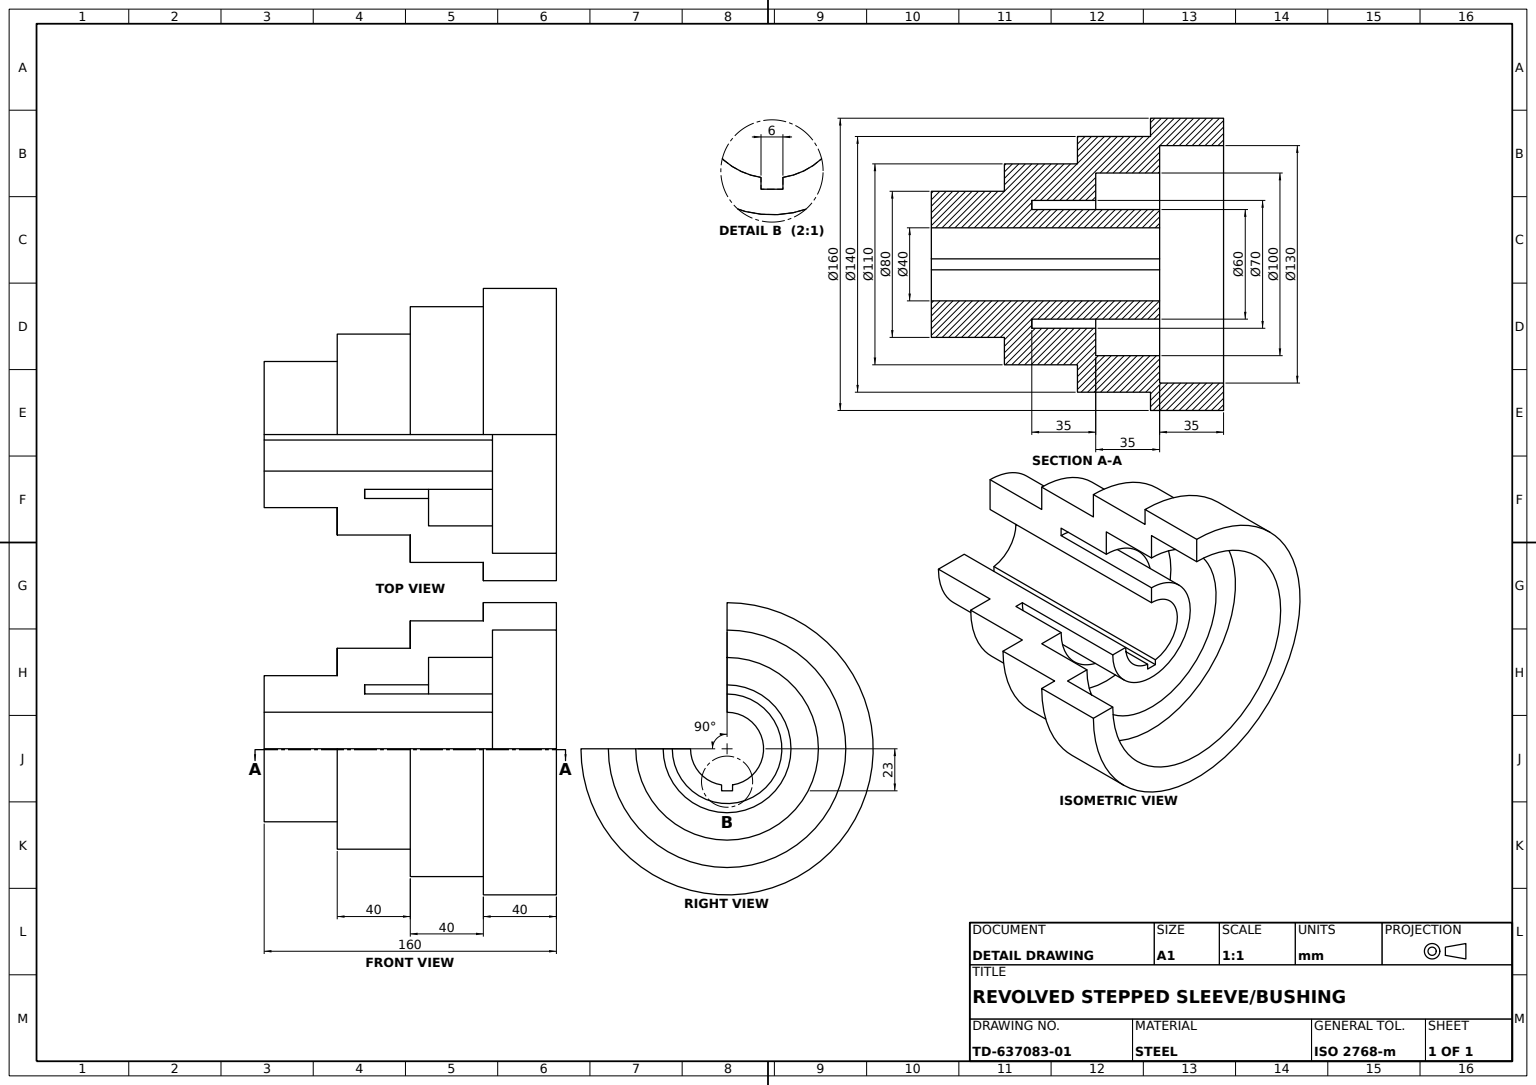
SolidWorks part; units mm, degrees
material "Plain Carbon Steel"
ref_plane "Front Plane" through (0, 0, 0) normal (0, 0, 1) x (1, 0, 0)
ref_plane "Top Plane" through (0, 0, 0) normal (0, 1, 0) x (1, 0, 0)
ref_plane "Right Plane" through (0, 0, 0) normal (1, 0, 0) x (0, 0, -1)
sketch "Pulley Profile Sketch" plane through (0, 0, 0) normal (0, 0, 1) x (1, 0, 0)
  line L0 (125, 0) -> (0, 0) construction
  line L1 (0, 0) -> (0, 40)
  line L2 (0, 40) -> (40, 40)
  line L3 (40, 40) -> (40, 55)
  line L4 (40, 55) -> (80, 55)
  line L5 (80, 55) -> (80, 70)
  line L6 (80, 70) -> (120, 70)
  line L7 (120, 70) -> (120, 80)
  line L8 (120, 80) -> (160, 80)
  line L9 (160, 80) -> (160, 65)
  line L10 (0, 20) -> (125, 20)
  line L11 (125, 20) -> (125, 30)
  line L12 (125, 30) -> (55, 30)
  line L13 (55, 30) -> (55, 35)
  line L14 (55, 35) -> (90, 35)
  line L15 (90, 35) -> (90, 50)
  line L16 (90, 50) -> (125, 50)
  line L17 (125, 50) -> (125, 65)
  line L18 (125, 65) -> (160, 65)
  line L19 (125, 20) -> (125, 0)
  dimension "D1" = 40
  dimension "D2" = 40
  dimension "D3" = 55
  dimension "D4" = 70
  dimension "D5" = 80
  dimension "D6" = 35
  dimension "D7" = 30
  dimension "D8" = 70
  dimension "D9" = 35
  dimension "D10" = 35
  dimension "D11" = 15
  dimension "D12" = 15
  dimension "D13" = 15
  dimension "D14" = 35
revolve "Stepped Pulley Body" add sketch "Pulley Profile Sketch" angle 270 about L0
sketch "Keyway Slot Sketch" plane through (0, 0, 0) normal (1, 0, 0) x (0, 0, -1)
  line L0 (0, 0) -> (0, -20) construction
  line L1 (0, -20) -> (0, -23)
  line L2 (0, -23) -> (3, -23)
  line L3 (3, -23) -> (3, -19.7737)
  line L5 (-3, -19.7737) -> (-3, -23)
  line L6 (-3, -23) -> (0, -23)
  line L7 (3, -19.7737) -> (-3, -19.7737)
  arc A0 (-20, 0) -> (0, 20) centre (0, 0) ccw construction
  arc A1 (-20, 0) -> (0, 20) centre (0, 0) ccw
  dimension "D1" = 6
  dimension "D2" = 3
extrude "Keyway Slot 6x3" cut sketch "Keyway Slot Sketch" against normal through all and the other way through all contours A1 L1 L2 L3 | A1 L5 L6 L1
